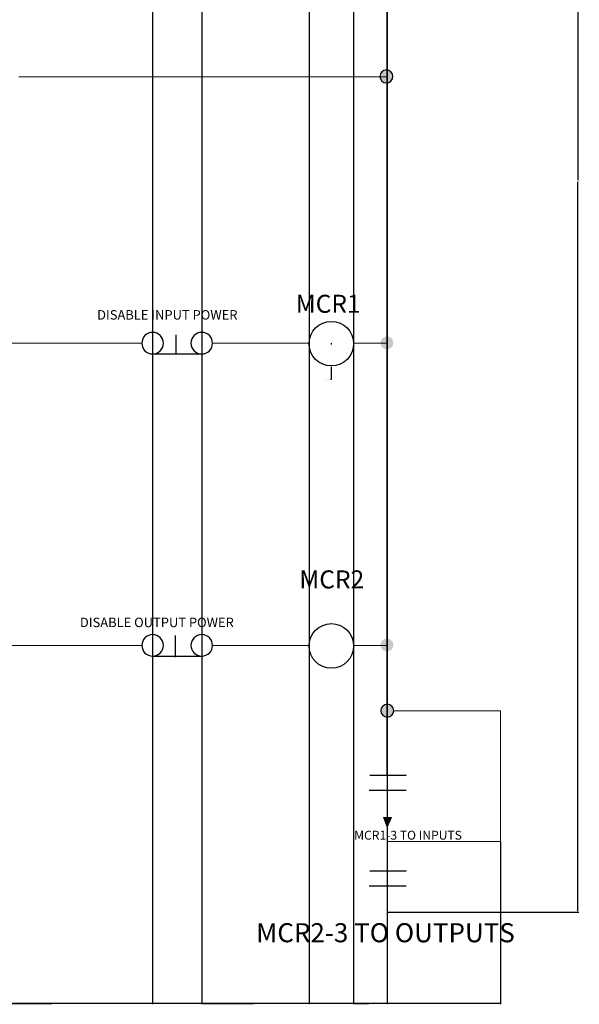
# Model space of a CAD drawing. Units: inches. Extents: x 738 to 1068, y 378 to 757.
# Tile 32 of 41: x 939 to 1068, y 378 to 606. Entities that reach past the tile are written whole.
import ezdxf

# ---------------------------------------------------------------- set-up
doc = ezdxf.new("R2010")
doc.units = ezdxf.units.IN
doc.header["$MEASUREMENT"] = 0
for name, color, linetype, lineweight in [('A-ANNO-DIMS', 2, 'Continuous', 18), ('E-ANNO-SYMB', 7, 'Continuous', 18), ('E-ANNO-TEXT', 7, 'Continuous', 18), ('E-CONN', 7, 'Continuous', 25), ('E-CONN-PATT', 7, 'Continuous', 13), ('E-CTRL-COIL', 4, 'Continuous', 25), ('E-CTRL-CONT', 4, 'Continuous', 25), ('E-CTRL-PBTN', 4, 'Continuous', 25), ('E-CTRL-WIRE', 7, 'Continuous', 18), ('E-POWR-FEED', 7, 'Continuous', 35)]:
    doc.layers.add(name, color=color, linetype=linetype, lineweight=lineweight)
doc.styles.get("Standard").update_dxf_attribs({"font": 'arial.ttf'})
doc.dimstyles.get("Standard").update_dxf_attribs({"dimtxt": 0.18, "dimasz": 0.18, "dimexe": 0.18, "dimexo": 0.0625, "dimgap": 0.09, "dimtad": 0, "dimtih": 1, "dimtoh": 1, "dimdec": 4, "dimzin": 0, "dimdsep": 46, "dimtxsty": 'Standard', "dimcen": 0.09, "dimadec": 0, "dimazin": 0, "dimtfac": 1, "dimtdec": 4, "dimtofl": 0, "dimtmove": 0, "dimatfit": 3, "dimfxl": 1, "dimtolj": 1, "dimtzin": 0, "dimarcsym": 0})

# ---------------------------------------------------------------- blocks, each defined once
blk = doc.blocks.new('RELAY-COIL')
blk.add_circle((5.16, 5.16), 5.16)
blk = doc.blocks.new('MCR-IO-CONTACT-NO')
for p, q in [((0.14, 3.47), (8.51, 3.47)), ((8.51, 3.47), (8.51, 3.54)), ((0, 0), (8.51, 0))]:
    blk.add_line(p, q)
blk = doc.blocks.new('FEED-CONTINUATION-ARROW')
h = blk.add_hatch(color=256)
h.dxf.hatch_style = 1
h.paths.add_polyline_path([(1.84, 2.25), (0, 2.25), (0.82, 0)])
for p, q in [((0, 2.25), (1.84, 2.25)), ((0.82, 0), (0, 2.25)), ((1.84, 2.25), (0.82, 0))]:
    blk.add_line(p, q)
blk = doc.blocks.new('*D17')
at = {"layer": 'A-ANNO-DIMS', "color": 0, "lineweight": -2, "transparency": 16777216}
for p, q in [((756.32, 415.84), (756.32, 378.24)), ((1050.05, 415.92), (1050.05, 378.24)), ((756.5, 378.42), (902.79, 378.42)), ((1049.87, 378.42), (903.58, 378.42))]:
    blk.add_line(p, q, dxfattribs=at)
at = {"layer": 'A-ANNO-DIMS', "color": 0, "transparency": 16777216}
for points in [[(756.5, 378.45), (756.5, 378.39), (756.32, 378.42)], [(1049.87, 378.45), (1049.87, 378.39), (1050.05, 378.42)]]:
    blk.add_solid(points, dxfattribs=at)
at = {"layer": 'Defpoints', "color": 0, "transparency": 16777216}
for p in [(756.32, 415.9), (1050.05, 415.98), (1050.05, 378.42)]:
    blk.add_point(p, dxfattribs=at)
at = {"layer": 'A-ANNO-DIMS', "color": 0, "transparency": 16777216, "insert": (903.19, 378.42), "char_height": 0.18, "attachment_point": 5}
blk.add_mtext('\\A1;293.7', dxfattribs=at)
blk = doc.blocks.new('*D18')
at = {"layer": 'A-ANNO-DIMS', "color": 0, "lineweight": -2, "transparency": 16777216}
for p, q in [((901.52, 738.38), (1068.18, 738.38)), ((1068, 738.2), (1068, 569.17)), ((1068, 399.78), (1068, 568.8)), ((1023.84, 399.6), (1068.18, 399.6))]:
    blk.add_line(p, q, dxfattribs=at)
at = {"layer": 'A-ANNO-DIMS', "color": 0, "transparency": 16777216}
for points in [[(1067.97, 738.2), (1068.03, 738.2), (1068, 738.38)], [(1067.97, 399.78), (1068.03, 399.78), (1068, 399.6)]]:
    blk.add_solid(points, dxfattribs=at)
at = {"layer": 'Defpoints', "color": 0, "transparency": 16777216}
for p in [(901.46, 738.38), (1068, 738.38), (1023.78, 399.6)]:
    blk.add_point(p, dxfattribs=at)
at = {"layer": 'A-ANNO-DIMS', "color": 0, "transparency": 16777216, "insert": (1068, 568.99), "char_height": 0.18, "attachment_point": 5}
blk.add_mtext('\\A1;338.8', dxfattribs=at)
blk = doc.blocks.new('*D28')
at = {"layer": 'A-ANNO-DIMS', "color": 0, "lineweight": -2, "transparency": 16777216}
for p, q in [((923.51, 646.92), (923.51, 378.24)), ((969.44, 646.92), (969.44, 378.24)), ((923.69, 378.42), (946.08, 378.42)), ((969.26, 378.42), (946.87, 378.42))]:
    blk.add_line(p, q, dxfattribs=at)
at = {"layer": 'A-ANNO-DIMS', "color": 0, "transparency": 16777216}
for points in [[(923.69, 378.45), (923.69, 378.39), (923.51, 378.42)], [(969.26, 378.45), (969.26, 378.39), (969.44, 378.42)]]:
    blk.add_solid(points, dxfattribs=at)
at = {"layer": 'Defpoints', "color": 0, "transparency": 16777216}
for p in [(923.51, 646.99), (969.44, 646.99), (969.44, 378.42)]:
    blk.add_point(p, dxfattribs=at)
at = {"layer": 'A-ANNO-DIMS', "color": 0, "transparency": 16777216, "insert": (946.48, 378.42), "char_height": 0.18, "attachment_point": 5}
blk.add_mtext('\\A1;45.93', dxfattribs=at)
blk = doc.blocks.new('*D29')
at = {"layer": 'A-ANNO-DIMS', "color": 0, "lineweight": -2, "transparency": 16777216}
for p, q in [((980.83, 646.92), (980.83, 378.24)), ((1005.69, 646.81), (1005.69, 378.24)), ((981.01, 378.42), (992.79, 378.42)), ((1005.51, 378.42), (993.72, 378.42))]:
    blk.add_line(p, q, dxfattribs=at)
at = {"layer": 'A-ANNO-DIMS', "color": 0, "transparency": 16777216}
for points in [[(981.01, 378.45), (981.01, 378.39), (980.83, 378.42)], [(1005.51, 378.45), (1005.51, 378.39), (1005.69, 378.42)]]:
    blk.add_solid(points, dxfattribs=at)
at = {"layer": 'Defpoints', "color": 0, "transparency": 16777216}
for p in [(980.83, 646.99), (1005.69, 646.87), (1005.69, 378.42)]:
    blk.add_point(p, dxfattribs=at)
at = {"layer": 'A-ANNO-DIMS', "color": 0, "transparency": 16777216, "insert": (993.26, 378.42), "char_height": 0.18, "attachment_point": 5}
blk.add_mtext('\\A1;24.864', dxfattribs=at)
blk = doc.blocks.new('*D30')
at = {"layer": 'A-ANNO-DIMS', "color": 0, "lineweight": -2, "transparency": 16777216}
for p, q in [((1016.01, 646.81), (1016.01, 378.24)), ((1023.82, 646.92), (1023.82, 378.24)), ((1016.19, 378.42), (1019.54, 378.42)), ((1023.64, 378.42), (1020.29, 378.42))]:
    blk.add_line(p, q, dxfattribs=at)
at = {"layer": 'A-ANNO-DIMS', "color": 0, "transparency": 16777216}
for points in [[(1016.19, 378.45), (1016.19, 378.39), (1016.01, 378.42)], [(1023.64, 378.45), (1023.64, 378.39), (1023.82, 378.42)]]:
    blk.add_solid(points, dxfattribs=at)
at = {"layer": 'Defpoints', "color": 0, "transparency": 16777216}
for p in [(1016.01, 646.87), (1023.82, 646.99), (1023.82, 378.42)]:
    blk.add_point(p, dxfattribs=at)
at = {"layer": 'A-ANNO-DIMS', "color": 0, "transparency": 16777216, "insert": (1019.92, 378.42), "char_height": 0.18, "attachment_point": 5}
blk.add_mtext('\\A1;7.811', dxfattribs=at)
blk = doc.blocks.new('*D42')
at = {"layer": 'A-ANNO-DIMS', "color": 0, "lineweight": -2, "transparency": 16777216}
for p, q in [((1010.76, 531.28), (1010.94, 531.28)), ((1010.85, 531.19), (1010.85, 531.37)), ((1010.85, 523.03), (1010.85, 525.94)), ((1010.67, 523.03), (1010.85, 523.03))]:
    blk.add_line(p, q, dxfattribs=at)
at = {"layer": 'A-ANNO-DIMS', "color": 0, "transparency": 16777216}
blk.add_solid([(1010.82, 525.94), (1010.88, 525.94), (1010.85, 526.12)], dxfattribs=at)
at = {"layer": 'Defpoints', "color": 0, "transparency": 16777216}
for p in [(1010.85, 536.45), (1010.85, 526.12)]:
    blk.add_point(p, dxfattribs=at)
at = {"layer": 'A-ANNO-DIMS', "color": 0, "transparency": 16777216, "insert": (1009.92, 523.03), "char_height": 0.18, "attachment_point": 5}
blk.add_mtext('\\A1;3X ∅10.323', dxfattribs=at)

msp = doc.modelspace()

# ---------------------------------------------------------------- hatches: boundary and pattern name
at = {"layer": 'E-CONN-PATT'}
h = msp.add_hatch(color=256, dxfattribs=at)
h.dxf.hatch_style = 1
h.paths.add_polyline_path([(781.4897, 594.5796, 0.41520307), (779.9846, 593.0796, 0.41520307), (781.4897, 591.5796)])
h.paths.add_polyline_path([(781.4897, 594.5796), (781.4897, 593.1296), (782.9838, 593.1296, 0.40350086)])
h.paths.add_polyline_path([(782.9846, 593.0796, 0.00833426), (782.9838, 593.1296), (781.4897, 593.1296), (781.4897, 591.5796, 0.41322475)])
h.paths.add_polyline_path([(1023.824, 594.6799), (1023.824, 591.7126, 0.37156792), (1025.1031, 593.1962, 0.37156792)])
h.paths.add_polyline_path([(1023.824, 593.1296), (1022.1046, 593.1296, 0.44481476), (1023.824, 591.7126)])
h.paths.add_polyline_path([(1023.824, 594.6799, 0.45818517), (1022.1031, 593.1962, 0.01110677), (1022.1046, 593.1296), (1023.824, 593.1296)])
h = msp.add_hatch(color=256, dxfattribs=at)
h.dxf.hatch_style = 1
h.paths.add_polyline_path([(1025.2273, 531.4724, 1), (1022.2273, 531.4724, 1)])
h = msp.add_hatch(color=256, dxfattribs=at)
h.dxf.hatch_style = 1
h.paths.add_polyline_path([(1025.2273, 461.4633, 1), (1022.2273, 461.4633, 1)])
h = msp.add_hatch(color=256, dxfattribs=at)
h.dxf.hatch_style = 1
h.paths.add_polyline_path([(1025.3162, 446.2651, 0.41322475), (1023.8213, 447.7651), (1023.8213, 444.7651, 0.41322475)])
h.paths.add_polyline_path([(1023.8213, 447.7651, 0.41520307), (1022.3162, 446.2651, 0.41520307), (1023.8213, 444.7651)])

# ---------------------------------------------------------------- linework, layer by layer
at = {"layer": 'E-CONN'}
for points in [[(1022.1031, 593.1962, 1), (1025.1031, 593.1962, 1)], [(1022.3162, 446.2651, 1), (1025.3162, 446.2651, 1)]]:
    msp.add_lwpolyline(points, format="xyb", close=True, dxfattribs=at)
at = {"layer": 'E-CTRL-PBTN'}
for p, q in [((974.9076, 528.7898), (974.9076, 533.3001)), ((969.4395, 528.9009), (980.8252, 528.9009)), ((974.7221, 458.6638), (974.7221, 463.6497)), ((969.4395, 458.8919), (980.8252, 458.8919))]:
    msp.add_line(p, q, dxfattribs=at)
for points in [[(966.9395, 531.4009, 1), (971.9395, 531.4009, 1)], [(978.3252, 531.4009, 1), (983.3252, 531.4009, 1)], [(966.9395, 461.3919, 1), (971.9395, 461.3919, 1)], [(978.3252, 461.3919, 1), (983.3252, 461.3919, 1)]]:
    msp.add_lwpolyline(points, format="xyb", close=True, dxfattribs=at)
at = {"layer": 'E-CTRL-WIRE'}
for p, q in [((938.455, 593.1296), (1023.824, 593.1296)), ((885.9574, 531.4009), (966.9395, 531.4009)), ((938.8276, 531.4009), (966.9395, 531.4009)), ((983.3252, 531.4009), (1005.6909, 531.4009)), ((1016.0116, 531.4009), (1023.824, 531.4009)), ((885.9574, 461.3919), (966.9395, 461.3919)), ((938.8276, 461.3919), (966.9395, 461.3919)), ((983.3252, 461.3919), (1005.6909, 461.3919)), ((1016.0116, 461.3919), (1023.824, 461.3919)), ((1025.3162, 446.2651), (1050.0492, 446.2651)), ((1050.0492, 446.2651), (1050.0492, 415.982)), ((1023.8213, 427.853), (1023.8213, 421.5166)), ((1023.779, 415.982), (1023.779, 409.1572)), ((1050.0492, 415.982), (1023.779, 415.982)), ((1023.779, 405.6894), (1023.779, 399.5952))]:
    msp.add_line(p, q, dxfattribs=at)
at = {"layer": 'E-POWR-FEED'}
for p, q in [((1023.824, 686.3292), (1023.824, 431.3208)), ((1023.8213, 437.8486), (1023.8213, 431.3208))]:
    msp.add_line(p, q, dxfattribs=at)

# ---------------------------------------------------------------- block references
at = {"layer": 'E-ANNO-SYMB'}
msp.add_blockref('FEED-CONTINUATION-ARROW', (1022.9596, 419.247), dxfattribs=at)
at = {"layer": 'E-CTRL-COIL'}
for p in [(1005.69, 526.1226), (1005.69, 456.1136)]:
    msp.add_blockref('RELAY-COIL', p, dxfattribs=at)
at = {"layer": 'E-CTRL-CONT'}
for p in [(1019.6426, 427.853), (1019.6426, 405.6894)]:
    msp.add_blockref('MCR-IO-CONTACT-NO', p, dxfattribs=at)

# ---------------------------------------------------------------- texts
at = {"layer": 'E-ANNO-TEXT'}
for s, height, p in [('MCR1', 4.17507, (1002.599, 538.4382)), ('DISABLE INPUT POWER ', 2.19392, (956.5783, 536.8705)), ('MCR2', 4.17507, (1003.4339, 474.5866)), ('DISABLE OUTPUT POWER', 2.19392, (952.5953, 465.618)), ('MCR1-3 TO INPUTS', 2.054977, (1016.1582, 416.3831)), ('MCR2-3 TO OUTPUTS', 4.418149, (993.4318, 392.6132))]:
    msp.add_text(s, height=height, dxfattribs=at).set_placement(p)

# ---------------------------------------------------------------- dimensions: what is measured, and where the dimension line sits
at = {"layer": 'A-ANNO-DIMS'}
dim = msp.add_linear_dim(base=(1067.9992, 738.3751), p1=(1023.779, 399.5952), p2=(901.4622, 738.3751), angle=90, dimstyle='Standard', override={"dimdec": 1, "dimlfac": 1, "dimrnd": 0, "dimzin": 0, "dimdsep": 46, "dimlunit": 2}, dxfattribs=at)
dim.commit()
dim.dimension.update_dxf_attribs({"geometry": '*D18', "text_midpoint": (1067.9992, 568.9851)})
for base, p1, p2, override, picture, middle in [((969.4395, 378.4191), (923.5105, 646.9853), (969.4395, 646.9853), {"dimdec": 2, "dimlfac": 1, "dimrnd": 0, "dimzin": 0, "dimdsep": 46, "dimlunit": 2}, '*D28', (946.475, 378.4191)), ((1005.6896, 378.4191), (980.8252, 646.9853), (1005.6896, 646.8683), {"dimdec": 3, "dimlfac": 1, "dimrnd": 0, "dimzin": 0, "dimdsep": 46, "dimlunit": 2}, '*D29', (993.2574, 378.4191)), ((1023.824, 378.4191), (1016.0129, 646.8683), (1023.824, 646.9853), {"dimdec": 3, "dimlfac": 1, "dimrnd": 0, "dimzin": 0, "dimdsep": 46, "dimlunit": 2}, '*D30', (1019.9185, 378.4191)), ((1050.0492, 378.4191), (756.3236, 415.904), (1050.0492, 415.982), {"dimdec": 1, "dimlfac": 1, "dimrnd": 0, "dimzin": 0, "dimdsep": 46, "dimlunit": 2}, '*D17', (903.1864, 378.4191))]:
    dim = msp.add_linear_dim(base=base, p1=p1, p2=p2, dimstyle='Standard', override=override, dxfattribs=at)
    dim.commit()
    dim.dimension.update_dxf_attribs({"geometry": picture, "text_midpoint": middle})
dim = msp.add_diameter_dim_2p(p1=(1010.8526, 536.4456), p2=(1010.85, 526.1223), text='3X <>', dimstyle='Standard', override={"dimdec": 3, "dimlfac": 1, "dimrnd": 0, "dimzin": 0, "dimdsep": 46, "dimlunit": 2}, dxfattribs=at)
dim.commit()
dim.dimension.update_dxf_attribs({"geometry": '*D42', "text_midpoint": (1009.9192, 523.0253), "dimtype": 163})

doc.saveas('drawing.dxf')
